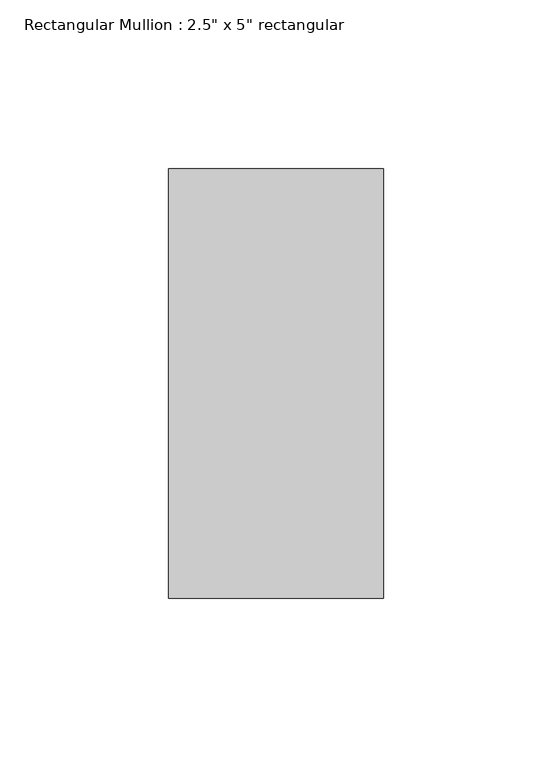
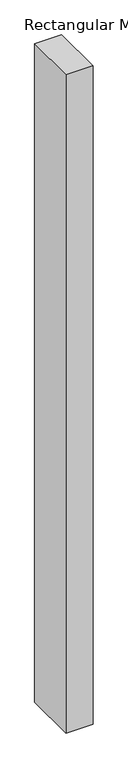
"""IFC4 building model written with IfcOpenShell, lengths in millimetres: member geometry."""

from ifc_helpers import new_model, si_unit, frame, origin, place, context, project, spatial, polyline, outline, extrude, source, transform, mapped, element, save


def member_f1c24713(model_context):
    return source(origin(), model_context, "Body", "SweptSolid", [
        extrude(outline(polyline([(0.0, 63.5), (0.0, -63.5), (-63.5, -63.5), (-63.5, 63.5), (0.0, 63.5)])), frame((0.0, 0.0, -1631.45108), z_axis=(0.0, 0.0, 1.0), x_axis=(1.0, 0.0, 0.0)), (0.0, 0.0, 1.0), 1631.45108),
    ])


if __name__ == "__main__":
    model = new_model("IFC4")
    model_context = context("Model", 3, world=origin())
    ifc_project = project(units=[si_unit("LENGTHUNIT", "METRE", prefix="MILLI")], contexts=[model_context])
    site = spatial("IfcSite", under=ifc_project)
    building = spatial("IfcBuilding", under=site)
    placement = place(None, origin())
    member_shape = member_f1c24713(model_context)
    element("IfcMember", 1, ObjectType="Rectangular Mullion : 2.5\" x 5\" rectangular", at=placement, inside=building, context=model_context, shape_type="MappedRepresentation", body=[
        mapped(member_shape, transform((0.0, 0.0, 0.0), x_axis=(1.0, 0.0, 0.0), y_axis=(0.0, 1.0, 0.0), z_axis=(0.0, 0.0, 1.0))),
    ])
    save(model, "model.ifc")

# Revit data of these elements
# Type "Rectangular Mullion : 2.5\" x 5\" rectangular"
#   built-in parameter 1007304 = 0.416667 (stored number, unit not read)
#   built-in parameter 1007301 = 0.104167 (stored number, unit not read)
#   built-in parameter 1007300 = 0.104167 (stored number, unit not read)
# Element 1 (IfcMember, "Rectangular Mullion : 2.5\" x 5\" rectangular")
#   Materials on its faces: "Aluminum"
# Materials
#   "Aluminum": class "Metal", colour RGB 247 247 247, transparency 0, Description = "Aluminum 6061", Cost = 0
